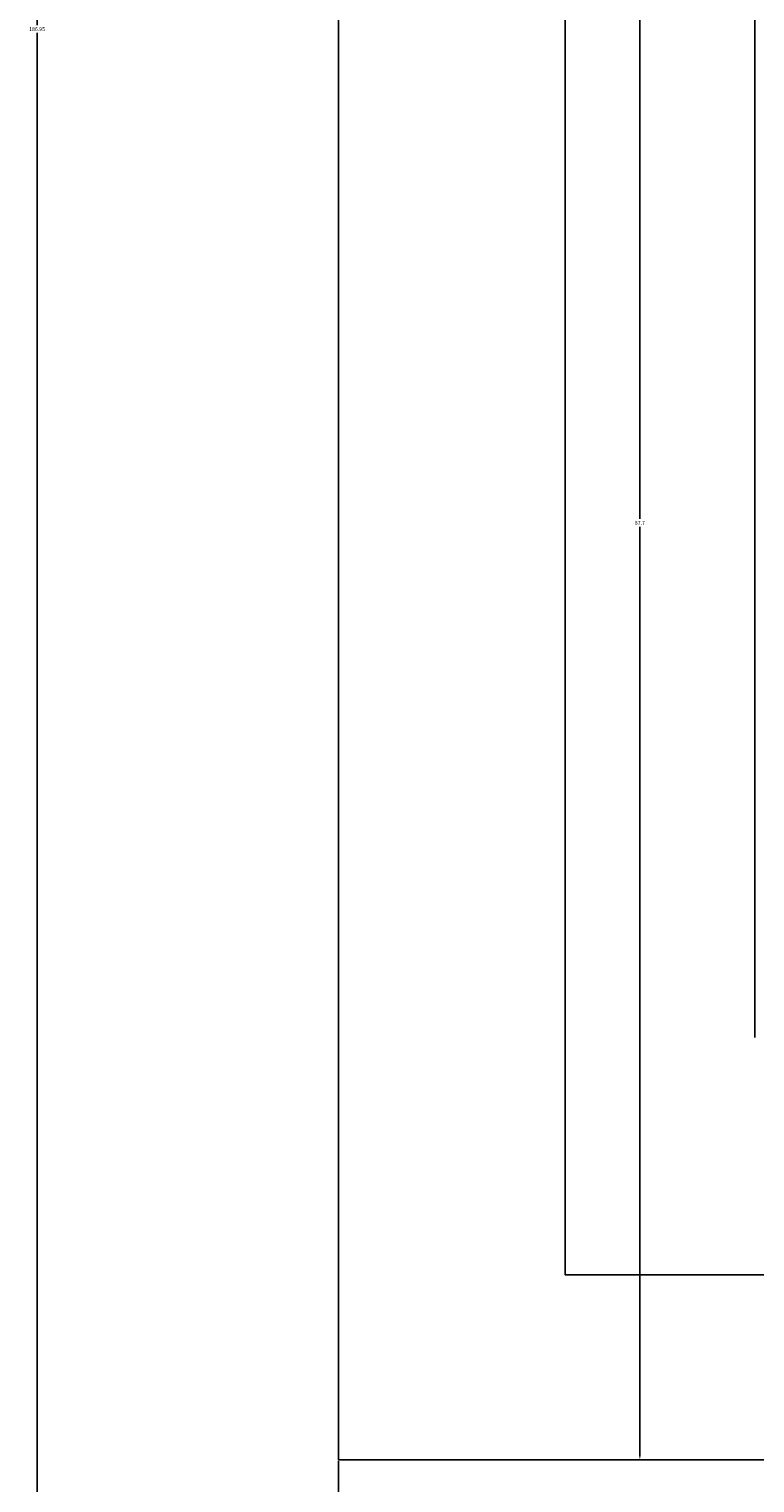
# Model space of a CAD drawing. Units: millimetres. Extents: x -8 to 285, y 5 to 221.
# Tile 4 of 30: x -8 to 26, y 45 to 113. Entities that reach past the tile are written whole.
import ezdxf

# ---------------------------------------------------------------- set-up
doc = ezdxf.new("R2010")
doc.units = ezdxf.units.MM
doc.layers.add('A-ANNO-DIMS', color=2, linetype='Continuous', lineweight=18)
doc.layers.add('E-POWR-DC-NEG', color=3, linetype='Continuous', lineweight=25)
doc.layers.add('E-POWR-DC-POS', color=30, linetype='Continuous', lineweight=25, true_color=0xf26722)
doc.styles.get("Standard").update_dxf_attribs({"font": 'arial.ttf'})
doc.dimstyles.get("Standard").update_dxf_attribs({"dimtxt": 0.18, "dimasz": 0.18, "dimexe": 0.18, "dimexo": 0.0625, "dimgap": 0.09, "dimtad": 0, "dimtih": 1, "dimtoh": 1, "dimdec": 4, "dimzin": 0, "dimdsep": 46, "dimtxsty": 'Standard', "dimcen": 0.09, "dimadec": 0, "dimazin": 0, "dimtfac": 1, "dimtdec": 4, "dimtofl": 0, "dimtmove": 0, "dimatfit": 3, "dimfxl": 1, "dimtolj": 1, "dimtzin": 0, "dimarcsym": 0})

# ---------------------------------------------------------------- blocks, each defined once
blk = doc.blocks.new('*D10')
at = {"layer": 'A-ANNO-DIMS', "color": 0, "lineweight": -2, "transparency": 16777216}
for p, q in [((145.103, 206.457), (-7.608, 206.457)), ((-7.428, 206.277), (-7.428, 113.161)), ((-7.428, 19.682), (-7.428, 112.797)), ((30.453, 19.502), (-7.608, 19.502))]:
    blk.add_line(p, q, dxfattribs=at)
at = {"layer": 'A-ANNO-DIMS', "color": 0, "transparency": 16777216}
for points in [[(-7.458, 206.277), (-7.398, 206.277), (-7.428, 206.457)], [(-7.458, 19.682), (-7.398, 19.682), (-7.428, 19.502)]]:
    blk.add_solid(points, dxfattribs=at)
at = {"layer": 'Defpoints', "color": 0, "transparency": 16777216}
for p in [(-7.428, 206.457), (145.165, 206.457), (30.516, 19.502)]:
    blk.add_point(p, dxfattribs=at)
at = {"layer": 'A-ANNO-DIMS', "color": 0, "transparency": 16777216, "insert": (-7.428, 112.979), "char_height": 0.18, "attachment_point": 5}
blk.add_mtext('\\A1;186.95', dxfattribs=at)
blk = doc.blocks.new('*D19')
at = {"layer": 'A-ANNO-DIMS', "color": 0, "lineweight": -2, "transparency": 16777216}
for p, q in [((6.735, 133.727), (20.952, 133.727)), ((20.772, 133.547), (20.772, 90.056)), ((20.772, 46.201), (20.772, 89.692)), ((6.735, 46.021), (20.952, 46.021))]:
    blk.add_line(p, q, dxfattribs=at)
at = {"layer": 'A-ANNO-DIMS', "color": 0, "transparency": 16777216}
for points in [[(20.742, 133.547), (20.802, 133.547), (20.772, 133.727)], [(20.742, 46.201), (20.802, 46.201), (20.772, 46.021)]]:
    blk.add_solid(points, dxfattribs=at)
at = {"layer": 'Defpoints', "color": 0, "transparency": 16777216}
for p in [(6.672, 133.727), (6.672, 46.021), (20.772, 46.021)]:
    blk.add_point(p, dxfattribs=at)
at = {"layer": 'A-ANNO-DIMS', "color": 0, "transparency": 16777216, "insert": (20.772, 89.874), "char_height": 0.18, "attachment_point": 5}
blk.add_mtext('\\A1;87.7', dxfattribs=at)
blk = doc.blocks.new('*D22')
at = {"layer": 'A-ANNO-DIMS', "color": 0, "lineweight": -2, "transparency": 16777216}
for p, q in [((6.672, 45.959), (6.672, 5.222)), ((30.516, 35.867), (30.516, 5.222)), ((6.852, 5.402), (18.129, 5.402)), ((30.336, 5.402), (19.059, 5.402))]:
    blk.add_line(p, q, dxfattribs=at)
at = {"layer": 'A-ANNO-DIMS', "color": 0, "transparency": 16777216}
for points in [[(6.852, 5.432), (6.852, 5.372), (6.672, 5.402)], [(30.336, 5.432), (30.336, 5.372), (30.516, 5.402)]]:
    blk.add_solid(points, dxfattribs=at)
at = {"layer": 'Defpoints', "color": 0, "transparency": 16777216}
for p in [(6.672, 46.021), (30.516, 35.929), (30.516, 5.402)]:
    blk.add_point(p, dxfattribs=at)
at = {"layer": 'A-ANNO-DIMS', "color": 0, "transparency": 16777216, "insert": (18.594, 5.402), "char_height": 0.18, "attachment_point": 5}
blk.add_mtext('\\A1;23.843', dxfattribs=at)
blk = doc.blocks.new('*D24')
at = {"layer": 'A-ANNO-DIMS', "color": 0, "lineweight": -2, "transparency": 16777216}
for p, q in [((6.672, 46.084), (6.672, 220.737)), ((6.852, 220.557), (15.959, 220.557)), ((25.975, 220.557), (16.869, 220.557)), ((26.155, 65.791), (26.155, 220.737))]:
    blk.add_line(p, q, dxfattribs=at)
at = {"layer": 'A-ANNO-DIMS', "color": 0, "transparency": 16777216}
for points in [[(6.852, 220.587), (6.852, 220.527), (6.672, 220.557)], [(25.975, 220.587), (25.975, 220.527), (26.155, 220.557)]]:
    blk.add_solid(points, dxfattribs=at)
at = {"layer": 'Defpoints', "color": 0, "transparency": 16777216}
for p in [(26.155, 220.557), (26.155, 65.728), (6.672, 46.021)]:
    blk.add_point(p, dxfattribs=at)
at = {"layer": 'A-ANNO-DIMS', "color": 0, "transparency": 16777216, "insert": (16.414, 220.557), "char_height": 0.18, "attachment_point": 5}
blk.add_mtext('\\A1;19.483', dxfattribs=at)

msp = doc.modelspace()

# ---------------------------------------------------------------- linework, layer by layer
at = {"layer": 'E-POWR-DC-NEG'}
msp.add_lwpolyline([(46.1717, 67.9064), (46.1717, 46.0211), (6.6725, 46.0211), (6.6725, 133.7273), (20.0566, 133.7273), (20.0566, 145.2715)], dxfattribs=at)
at = {"layer": 'E-POWR-DC-POS'}
msp.add_lwpolyline([(74.9801, 145.2715), (74.9801, 123.1618), (17.279, 123.1618), (17.279, 54.6776), (40.1717, 54.6776), (40.1717, 67.9064)], dxfattribs=at)

# ---------------------------------------------------------------- dimensions: what is measured, and where the dimension line sits
at = {"layer": 'A-ANNO-DIMS'}
for base, p1, p2, picture, middle in [((26.1554, 220.5568), (6.6725, 46.0211), (26.1554, 65.7282), '*D24', (16.4139, 220.5568)), ((30.51597, 5.40199), (6.67248, 46.02115), (30.51597, 35.92922), '*D22', (18.59423, 5.40199))]:
    dim = msp.add_linear_dim(base=base, p1=p1, p2=p2, dimstyle='Standard', override={"dimdec": 3, "dimlfac": 1, "dimrnd": 0, "dimzin": 0, "dimdsep": 46, "dimlunit": 2}, dxfattribs=at)
    dim.commit()
    dim.dimension.update_dxf_attribs({"geometry": picture, "text_midpoint": middle})
for base, p1, p2, angle, override, picture, middle in [((-7.4275, 206.4568), (30.516, 19.502), (145.1651, 206.4568), 90, {"dimdec": 2, "dimlfac": 1, "dimrnd": 0, "dimzin": 0, "dimdsep": 46, "dimlunit": 2}, '*D10', (-7.4275, 112.9794)), ((20.7725, 46.0211), (6.6725, 133.7273), (6.6725, 46.0211), 270, {"dimdec": 1, "dimlfac": 1, "dimrnd": 0, "dimzin": 0, "dimdsep": 46, "dimlunit": 2}, '*D19', (20.7725, 89.8742))]:
    dim = msp.add_linear_dim(base=base, p1=p1, p2=p2, angle=angle, dimstyle='Standard', override=override, dxfattribs=at)
    dim.commit()
    dim.dimension.update_dxf_attribs({"geometry": picture, "text_midpoint": middle})

doc.saveas('drawing.dxf')
